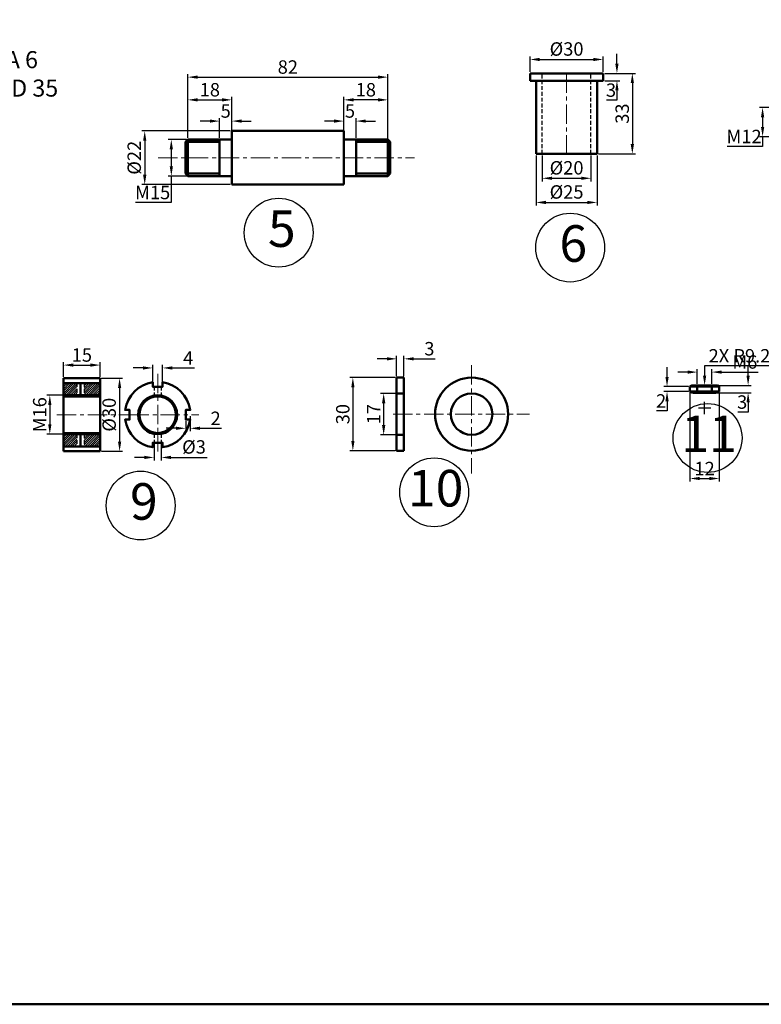
# Model space of a CAD drawing. Units: millimetres. Extents: x -3 to 930, y -425 to 322.
# Tile 2 of 5: x 225 to 529, y -425 to -21. Entities that reach past the tile are written whole.
import ezdxf
from ezdxf import colors
from ezdxf.entities.mleader import LeaderData, LeaderLine
from ezdxf.math import Vec2, Vec3

# ---------------------------------------------------------------- set-up
doc = ezdxf.new("R2010")
doc.units = ezdxf.units.MM
doc.header["$LTSCALE"] = 0.5
doc.linetypes.add('CENTER', pattern=[50.8, 31.75, -6.35, 6.35, -6.35])
doc.linetypes.add('HIDDEN', pattern=[9.525, 6.35, -3.175])
for name, color, linetype, lineweight in [('M-ANNO-SYMB', 3, 'Continuous', 25), ('M-CNTR', 1, 'CENTER', 18), ('M-DIMS', 2, 'Continuous', 25), ('M-HATC', 8, 'Continuous', 18), ('M-HIDN', 4, 'HIDDEN', 25), ('M-OUTL', 7, 'Continuous', 50), ('M-TEXT', 3, 'Continuous', 25)]:
    doc.layers.add(name, color=color, linetype=linetype, lineweight=lineweight)
doc.styles.get("Standard").update_dxf_attribs({"font": 'arial.ttf'})
doc.dimstyles.new('ISO-25', dxfattribs={"dimtxt": 5.5, "dimasz": 4, "dimexe": 1.25, "dimexo": 0.625, "dimtad": 1, "dimtoh": 1, "dimdec": 0, "dimtxsty": 'Standard', "dimcen": 2.5, "dimadec": 0, "dimazin": 0, "dimtfac": 1, "dimtdec": 0, "dimtofl": 0, "dimtmove": 0, "dimatfit": 3, "dimfxl": 1, "dimarcsym": 0})

# ---------------------------------------------------------------- blocks, each defined once
blk = doc.blocks.new('*D49')
at = {"layer": 'Defpoints', "color": 0, "ltscale": 0.5, "transparency": 16777216}
for p in [(311.91, -62.44), (306.91, -69.98), (311.91, -69.98)]:
    blk.add_point(p, dxfattribs=at)
at = {"layer": 'M-DIMS', "color": 0, "lineweight": -2, "ltscale": 0.5, "transparency": 16777216}
for p, q in [((302.91, -62.44), (298.91, -62.44)), ((306.91, -69.36), (306.91, -61.19)), ((311.91, -69.36), (311.91, -61.19)), ((315.91, -62.44), (319.91, -62.44))]:
    blk.add_line(p, q, dxfattribs=at)
at = {"layer": 'M-DIMS', "color": 0, "ltscale": 0.5, "transparency": 16777216}
for points in [[(302.91, -61.77), (302.91, -63.1), (306.91, -62.44)], [(315.91, -61.77), (315.91, -63.1), (311.91, -62.44)]]:
    blk.add_solid(points, dxfattribs=at)
at = {"layer": 'M-DIMS', "color": 0, "ltscale": 0.5, "transparency": 16777216, "insert": (309.41, -59.01), "char_height": 5.5, "attachment_point": 5}
blk.add_mtext('5', dxfattribs=at)
blk = doc.blocks.new('*D50')
at = {"layer": 'Defpoints', "color": 0, "ltscale": 0.5, "transparency": 16777216}
for p in [(311.91, -53.72), (293.91, -69.98), (311.91, -69.98)]:
    blk.add_point(p, dxfattribs=at)
at = {"layer": 'M-DIMS', "color": 0, "lineweight": -2, "ltscale": 0.5, "transparency": 16777216}
for p, q in [((293.91, -69.36), (293.91, -52.47)), ((311.91, -69.36), (311.91, -52.47)), ((297.91, -53.72), (307.91, -53.72))]:
    blk.add_line(p, q, dxfattribs=at)
at = {"layer": 'M-DIMS', "color": 0, "ltscale": 0.5, "transparency": 16777216}
for points in [[(297.91, -53.06), (297.91, -54.39), (293.91, -53.72)], [(307.91, -53.06), (307.91, -54.39), (311.91, -53.72)]]:
    blk.add_solid(points, dxfattribs=at)
at = {"layer": 'M-DIMS', "color": 0, "ltscale": 0.5, "transparency": 16777216, "insert": (302.91, -50.29), "char_height": 5.5, "attachment_point": 5}
blk.add_mtext('18', dxfattribs=at)
blk = doc.blocks.new('*D51')
at = {"layer": 'Defpoints', "color": 0, "ltscale": 0.5, "transparency": 16777216}
for p in [(375.91, -44.4), (293.91, -58.17), (375.91, -70.98)]:
    blk.add_point(p, dxfattribs=at)
at = {"layer": 'M-DIMS', "color": 0, "lineweight": -2, "ltscale": 0.5, "transparency": 16777216}
for p, q in [((293.91, -57.54), (293.91, -43.15)), ((297.91, -44.4), (371.91, -44.4)), ((375.91, -70.36), (375.91, -43.15))]:
    blk.add_line(p, q, dxfattribs=at)
at = {"layer": 'M-DIMS', "color": 0, "ltscale": 0.5, "transparency": 16777216}
for points in [[(297.91, -43.73), (297.91, -45.06), (293.91, -44.4)], [(371.91, -43.73), (371.91, -45.06), (375.91, -44.4)]]:
    blk.add_solid(points, dxfattribs=at)
at = {"layer": 'M-DIMS', "color": 0, "ltscale": 0.5, "transparency": 16777216, "insert": (334.91, -40.96), "char_height": 5.5, "attachment_point": 5}
blk.add_mtext('82', dxfattribs=at)
blk = doc.blocks.new('*D52')
at = {"layer": 'Defpoints', "color": 0, "ltscale": 0.5, "transparency": 16777216}
for p in [(311.91, -66.48), (276.18, -88.48), (311.91, -88.48)]:
    blk.add_point(p, dxfattribs=at)
at = {"layer": 'M-DIMS', "color": 0, "lineweight": -2, "ltscale": 0.5, "transparency": 16777216}
for p, q in [((311.28, -66.48), (274.93, -66.48)), ((276.18, -70.48), (276.18, -84.48)), ((311.28, -88.48), (274.93, -88.48))]:
    blk.add_line(p, q, dxfattribs=at)
at = {"layer": 'M-DIMS', "color": 0, "ltscale": 0.5, "transparency": 16777216}
for points in [[(275.51, -70.48), (276.85, -70.48), (276.18, -66.48)], [(275.51, -84.48), (276.85, -84.48), (276.18, -88.48)]]:
    blk.add_solid(points, dxfattribs=at)
at = {"layer": 'M-DIMS', "color": 0, "ltscale": 0.5, "transparency": 16777216, "insert": (272.59, -77.48), "char_height": 5.5, "attachment_point": 5, "rotation": 90}
blk.add_mtext('%%C22', dxfattribs=at)
blk = doc.blocks.new('*D53')
at = {"layer": 'Defpoints', "color": 0, "ltscale": 0.5, "transparency": 16777216}
for p in [(293.91, -69.98), (287.09, -84.98), (293.91, -84.98)]:
    blk.add_point(p, dxfattribs=at)
at = {"layer": 'M-DIMS', "color": 0, "lineweight": -2, "ltscale": 0.5, "transparency": 16777216}
for p, q in [((293.28, -69.98), (285.84, -69.98)), ((287.09, -73.98), (287.09, -80.98)), ((293.28, -84.98), (285.84, -84.98)), ((287.09, -84.98), (287.09, -95.89)), ((287.09, -95.89), (272.4, -95.89))]:
    blk.add_line(p, q, dxfattribs=at)
at = {"layer": 'M-DIMS', "color": 0, "ltscale": 0.5, "transparency": 16777216}
for points in [[(286.43, -73.98), (287.76, -73.98), (287.09, -69.98)], [(286.43, -80.98), (287.76, -80.98), (287.09, -84.98)]]:
    blk.add_solid(points, dxfattribs=at)
at = {"layer": 'M-DIMS', "color": 0, "ltscale": 0.5, "transparency": 16777216, "insert": (279.43, -92.46), "char_height": 5.5, "width": 8.2937, "attachment_point": 5}
blk.add_mtext('M15', dxfattribs=at)
blk = doc.blocks.new('*D54')
at = {"layer": 'Defpoints', "color": 0, "ltscale": 0.5, "transparency": 16777216}
for p in [(357.91, -62.44), (357.91, -69.98), (362.91, -69.98)]:
    blk.add_point(p, dxfattribs=at)
at = {"layer": 'M-DIMS', "color": 0, "lineweight": -2, "ltscale": 0.5, "transparency": 16777216}
for p, q in [((353.91, -62.44), (349.91, -62.44)), ((357.91, -69.36), (357.91, -61.19)), ((362.91, -69.36), (362.91, -61.19)), ((366.91, -62.44), (370.91, -62.44))]:
    blk.add_line(p, q, dxfattribs=at)
at = {"layer": 'M-DIMS', "color": 0, "ltscale": 0.5, "transparency": 16777216}
for points in [[(353.91, -61.77), (353.91, -63.1), (357.91, -62.44)], [(366.91, -61.77), (366.91, -63.1), (362.91, -62.44)]]:
    blk.add_solid(points, dxfattribs=at)
at = {"layer": 'M-DIMS', "color": 0, "ltscale": 0.5, "transparency": 16777216, "insert": (360.41, -59.01), "char_height": 5.5, "attachment_point": 5}
blk.add_mtext('5', dxfattribs=at)
blk = doc.blocks.new('*D55')
at = {"layer": 'Defpoints', "color": 0, "ltscale": 0.5, "transparency": 16777216}
for p in [(357.91, -53.72), (357.91, -69.98), (375.91, -69.98)]:
    blk.add_point(p, dxfattribs=at)
at = {"layer": 'M-DIMS', "color": 0, "lineweight": -2, "ltscale": 0.5, "transparency": 16777216}
for p, q in [((357.91, -69.36), (357.91, -52.47)), ((375.91, -69.36), (375.91, -52.47)), ((371.91, -53.72), (361.91, -53.72))]:
    blk.add_line(p, q, dxfattribs=at)
at = {"layer": 'M-DIMS', "color": 0, "ltscale": 0.5, "transparency": 16777216}
for points in [[(361.91, -53.06), (361.91, -54.39), (357.91, -53.72)], [(371.91, -53.06), (371.91, -54.39), (375.91, -53.72)]]:
    blk.add_solid(points, dxfattribs=at)
at = {"layer": 'M-DIMS', "color": 0, "ltscale": 0.5, "transparency": 16777216, "insert": (366.91, -50.29), "char_height": 5.5, "attachment_point": 5}
blk.add_mtext('18', dxfattribs=at)
blk = doc.blocks.new('*D56')
at = {"layer": 'Defpoints', "color": 0, "ltscale": 0.5, "transparency": 16777216}
for p in [(464.29, -42.87), (464.29, -45.87), (469.95, -45.87)]:
    blk.add_point(p, dxfattribs=at)
at = {"layer": 'M-DIMS', "color": 0, "lineweight": -2, "ltscale": 0.5, "transparency": 16777216}
for p, q in [((469.95, -38.87), (469.95, -34.87)), ((464.92, -42.87), (471.2, -42.87)), ((464.92, -45.87), (471.2, -45.87)), ((469.95, -49.87), (469.95, -53.87)), ((469.95, -53.87), (465.72, -53.87))]:
    blk.add_line(p, q, dxfattribs=at)
at = {"layer": 'M-DIMS', "color": 0, "ltscale": 0.5, "transparency": 16777216}
for points in [[(469.28, -38.87), (470.62, -38.87), (469.95, -42.87)], [(469.28, -49.87), (470.62, -49.87), (469.95, -45.87)]]:
    blk.add_solid(points, dxfattribs=at)
at = {"layer": 'M-DIMS', "color": 0, "ltscale": 0.5, "transparency": 16777216, "insert": (467.52, -50.43), "char_height": 5.5, "attachment_point": 5}
blk.add_mtext('3', dxfattribs=at)
blk = doc.blocks.new('*D57')
at = {"layer": 'Defpoints', "color": 0, "ltscale": 0.5, "transparency": 16777216}
for p in [(464.29, -42.87), (461.79, -75.87), (476.27, -75.87)]:
    blk.add_point(p, dxfattribs=at)
at = {"layer": 'M-DIMS', "color": 0, "lineweight": -2, "ltscale": 0.5, "transparency": 16777216}
for p, q in [((464.92, -42.87), (477.52, -42.87)), ((476.27, -46.87), (476.27, -71.87)), ((462.42, -75.87), (477.52, -75.87))]:
    blk.add_line(p, q, dxfattribs=at)
at = {"layer": 'M-DIMS', "color": 0, "ltscale": 0.5, "transparency": 16777216}
for points in [[(475.6, -46.87), (476.94, -46.87), (476.27, -42.87)], [(475.6, -71.87), (476.94, -71.87), (476.27, -75.87)]]:
    blk.add_solid(points, dxfattribs=at)
at = {"layer": 'M-DIMS', "color": 0, "ltscale": 0.5, "transparency": 16777216, "insert": (472.83, -59.37), "char_height": 5.5, "attachment_point": 5, "rotation": 90}
blk.add_mtext('33', dxfattribs=at)
blk = doc.blocks.new('*D58')
at = {"layer": 'Defpoints', "color": 0, "ltscale": 0.5, "transparency": 16777216}
for p in [(439.29, -75.87), (459.29, -75.87), (459.29, -85.91)]:
    blk.add_point(p, dxfattribs=at)
at = {"layer": 'M-DIMS', "color": 0, "lineweight": -2, "ltscale": 0.5, "transparency": 16777216}
for p, q in [((439.29, -76.49), (439.29, -87.16)), ((459.29, -76.49), (459.29, -87.16)), ((443.29, -85.91), (455.29, -85.91))]:
    blk.add_line(p, q, dxfattribs=at)
at = {"layer": 'M-DIMS', "color": 0, "ltscale": 0.5, "transparency": 16777216}
for points in [[(443.29, -85.24), (443.29, -86.57), (439.29, -85.91)], [(455.29, -85.24), (455.29, -86.57), (459.29, -85.91)]]:
    blk.add_solid(points, dxfattribs=at)
at = {"layer": 'M-DIMS', "color": 0, "ltscale": 0.5, "transparency": 16777216, "insert": (449.29, -82.32), "char_height": 5.5, "attachment_point": 5}
blk.add_mtext('%%C20', dxfattribs=at)
blk = doc.blocks.new('*D59')
at = {"layer": 'Defpoints', "color": 0, "ltscale": 0.5, "transparency": 16777216}
for p in [(436.79, -75.87), (461.79, -75.87), (461.79, -95.82)]:
    blk.add_point(p, dxfattribs=at)
at = {"layer": 'M-DIMS', "color": 0, "lineweight": -2, "ltscale": 0.5, "transparency": 16777216}
for p, q in [((436.79, -76.49), (436.79, -97.07)), ((461.79, -76.49), (461.79, -97.07)), ((440.79, -95.82), (457.79, -95.82))]:
    blk.add_line(p, q, dxfattribs=at)
at = {"layer": 'M-DIMS', "color": 0, "ltscale": 0.5, "transparency": 16777216}
for points in [[(440.79, -95.15), (440.79, -96.49), (436.79, -95.82)], [(457.79, -95.15), (457.79, -96.49), (461.79, -95.82)]]:
    blk.add_solid(points, dxfattribs=at)
at = {"layer": 'M-DIMS', "color": 0, "ltscale": 0.5, "transparency": 16777216, "insert": (449.29, -92.23), "char_height": 5.5, "attachment_point": 5}
blk.add_mtext('%%C25', dxfattribs=at)
blk = doc.blocks.new('*D60')
at = {"layer": 'Defpoints', "color": 0, "ltscale": 0.5, "transparency": 16777216}
for p in [(464.29, -37.15), (434.29, -42.87), (464.29, -42.87)]:
    blk.add_point(p, dxfattribs=at)
at = {"layer": 'M-DIMS', "color": 0, "lineweight": -2, "ltscale": 0.5, "transparency": 16777216}
for p, q in [((434.29, -42.24), (434.29, -35.9)), ((464.29, -42.24), (464.29, -35.9)), ((438.29, -37.15), (460.29, -37.15))]:
    blk.add_line(p, q, dxfattribs=at)
at = {"layer": 'M-DIMS', "color": 0, "ltscale": 0.5, "transparency": 16777216}
for points in [[(438.29, -36.48), (438.29, -37.82), (434.29, -37.15)], [(460.29, -36.48), (460.29, -37.82), (464.29, -37.15)]]:
    blk.add_solid(points, dxfattribs=at)
at = {"layer": 'M-DIMS', "color": 0, "ltscale": 0.5, "transparency": 16777216, "insert": (449.29, -33.56), "char_height": 5.5, "attachment_point": 5}
blk.add_mtext('%%C30', dxfattribs=at)
blk = doc.blocks.new('*D66')
at = {"layer": 'Defpoints', "color": 0, "ltscale": 0.5, "transparency": 16777216}
for p in [(257.89, -167.94), (257.89, -197.94), (265.87, -197.94)]:
    blk.add_point(p, dxfattribs=at)
at = {"layer": 'M-DIMS', "color": 0, "lineweight": -2, "ltscale": 0.5, "transparency": 16777216}
for p, q in [((258.51, -167.94), (267.12, -167.94)), ((265.87, -171.94), (265.87, -193.94)), ((258.51, -197.94), (267.12, -197.94))]:
    blk.add_line(p, q, dxfattribs=at)
at = {"layer": 'M-DIMS', "color": 0, "ltscale": 0.5, "transparency": 16777216}
for points in [[(265.21, -171.94), (266.54, -171.94), (265.87, -167.94)], [(265.21, -193.94), (266.54, -193.94), (265.87, -197.94)]]:
    blk.add_solid(points, dxfattribs=at)
at = {"layer": 'M-DIMS', "color": 0, "ltscale": 0.5, "transparency": 16777216, "insert": (262.29, -182.94), "char_height": 5.5, "attachment_point": 5, "rotation": 90}
blk.add_mtext('%%C30', dxfattribs=at)
blk = doc.blocks.new('*D67')
at = {"layer": 'Defpoints', "color": 0, "ltscale": 0.5, "transparency": 16777216}
for p in [(257.89, -162.57), (242.89, -167.94), (257.89, -167.94)]:
    blk.add_point(p, dxfattribs=at)
at = {"layer": 'M-DIMS', "color": 0, "lineweight": -2, "ltscale": 0.5, "transparency": 16777216}
for p, q in [((242.89, -167.32), (242.89, -161.32)), ((257.89, -167.32), (257.89, -161.32)), ((246.89, -162.57), (253.89, -162.57))]:
    blk.add_line(p, q, dxfattribs=at)
at = {"layer": 'M-DIMS', "color": 0, "ltscale": 0.5, "transparency": 16777216}
for points in [[(246.89, -161.9), (246.89, -163.24), (242.89, -162.57)], [(253.89, -161.9), (253.89, -163.24), (257.89, -162.57)]]:
    blk.add_solid(points, dxfattribs=at)
at = {"layer": 'M-DIMS', "color": 0, "ltscale": 0.5, "transparency": 16777216, "insert": (250.39, -159.14), "char_height": 5.5, "attachment_point": 5}
blk.add_mtext('15', dxfattribs=at)
blk = doc.blocks.new('*D68')
at = {"layer": 'Defpoints', "color": 0, "ltscale": 0.5, "transparency": 16777216}
for p in [(242.89, -174.94), (237.24, -190.94), (242.89, -190.94)]:
    blk.add_point(p, dxfattribs=at)
at = {"layer": 'M-DIMS', "color": 0, "lineweight": -2, "ltscale": 0.5, "transparency": 16777216}
for p, q in [((242.26, -174.94), (235.99, -174.94)), ((237.24, -178.94), (237.24, -186.94)), ((242.26, -190.94), (235.99, -190.94))]:
    blk.add_line(p, q, dxfattribs=at)
at = {"layer": 'M-DIMS', "color": 0, "ltscale": 0.5, "transparency": 16777216}
for points in [[(236.57, -178.94), (237.9, -178.94), (237.24, -174.94)], [(236.57, -186.94), (237.9, -186.94), (237.24, -190.94)]]:
    blk.add_solid(points, dxfattribs=at)
at = {"layer": 'M-DIMS', "color": 0, "ltscale": 0.5, "transparency": 16777216, "insert": (233.8, -182.94), "char_height": 5.5, "attachment_point": 5, "rotation": 90}
blk.add_mtext('M16', dxfattribs=at)
blk = doc.blocks.new('*D69')
at = {"layer": 'Defpoints', "color": 0, "ltscale": 0.5, "transparency": 16777216}
for p in [(283.49, -163.74), (279.49, -171.44), (283.49, -171.44)]:
    blk.add_point(p, dxfattribs=at)
at = {"layer": 'M-DIMS', "color": 0, "lineweight": -2, "ltscale": 0.5, "transparency": 16777216}
for p, q in [((275.49, -163.74), (271.49, -163.74)), ((279.49, -170.82), (279.49, -162.49)), ((283.49, -170.82), (283.49, -162.49)), ((287.49, -163.74), (296.55, -163.74))]:
    blk.add_line(p, q, dxfattribs=at)
at = {"layer": 'M-DIMS', "color": 0, "ltscale": 0.5, "transparency": 16777216}
for points in [[(275.49, -163.08), (275.49, -164.41), (279.49, -163.74)], [(287.49, -163.08), (287.49, -164.41), (283.49, -163.74)]]:
    blk.add_solid(points, dxfattribs=at)
at = {"layer": 'M-DIMS', "color": 0, "ltscale": 0.5, "transparency": 16777216, "insert": (294.02, -160.37), "char_height": 5.5, "attachment_point": 5}
blk.add_mtext('4', dxfattribs=at)
blk = doc.blocks.new('*D70')
at = {"layer": 'Defpoints', "color": 0, "ltscale": 0.5, "transparency": 16777216}
for p in [(279.99, -194.44), (282.99, -194.44), (282.99, -200.46)]:
    blk.add_point(p, dxfattribs=at)
at = {"layer": 'M-DIMS', "color": 0, "lineweight": -2, "ltscale": 0.5, "transparency": 16777216}
for p, q in [((279.99, -195.07), (279.99, -201.71)), ((282.99, -195.07), (282.99, -201.71)), ((275.99, -200.46), (271.99, -200.46)), ((286.99, -200.46), (301.83, -200.46))]:
    blk.add_line(p, q, dxfattribs=at)
at = {"layer": 'M-DIMS', "color": 0, "ltscale": 0.5, "transparency": 16777216}
for points in [[(275.99, -199.79), (275.99, -201.13), (279.99, -200.46)], [(286.99, -199.79), (286.99, -201.13), (282.99, -200.46)]]:
    blk.add_solid(points, dxfattribs=at)
at = {"layer": 'M-DIMS', "color": 0, "ltscale": 0.5, "transparency": 16777216, "insert": (296.41, -196.87), "char_height": 5.5, "attachment_point": 5}
blk.add_mtext('%%C3', dxfattribs=at)
blk = doc.blocks.new('*D71')
at = {"layer": 'Defpoints', "color": 0, "ltscale": 0.5, "transparency": 16777216}
for p in [(292.99, -184.94), (294.84, -182.94), (294.84, -188.5)]:
    blk.add_point(p, dxfattribs=at)
at = {"layer": 'M-DIMS', "color": 0, "lineweight": -2, "ltscale": 0.5, "transparency": 16777216}
for p, q in [((292.99, -185.57), (292.99, -189.75)), ((294.84, -183.57), (294.84, -189.75)), ((288.99, -188.5), (284.99, -188.5)), ((298.84, -188.5), (307.74, -188.5))]:
    blk.add_line(p, q, dxfattribs=at)
at = {"layer": 'M-DIMS', "color": 0, "ltscale": 0.5, "transparency": 16777216}
for points in [[(288.99, -187.83), (288.99, -189.17), (292.99, -188.5)], [(298.84, -187.83), (298.84, -189.17), (294.84, -188.5)]]:
    blk.add_solid(points, dxfattribs=at)
at = {"layer": 'M-DIMS', "color": 0, "ltscale": 0.5, "transparency": 16777216, "insert": (305.29, -185.12), "char_height": 5.5, "attachment_point": 5}
blk.add_mtext('2', dxfattribs=at)
blk = doc.blocks.new('*D75')
at = {"layer": 'Defpoints', "color": 0, "ltscale": 0.5, "transparency": 16777216}
for p in [(539.21, -56.85), (529.72, -68.85), (539.21, -68.85)]:
    blk.add_point(p, dxfattribs=at)
at = {"layer": 'M-DIMS', "color": 0, "lineweight": -2, "ltscale": 0.5, "transparency": 16777216}
for p, q in [((538.59, -56.85), (528.47, -56.85)), ((529.72, -60.85), (529.72, -64.85)), ((538.59, -68.85), (528.47, -68.85)), ((529.72, -68.85), (529.72, -72.85)), ((529.72, -72.85), (515.13, -72.85))]:
    blk.add_line(p, q, dxfattribs=at)
at = {"layer": 'M-DIMS', "color": 0, "ltscale": 0.5, "transparency": 16777216}
for points in [[(529.06, -60.85), (530.39, -60.85), (529.72, -56.85)], [(529.06, -64.85), (530.39, -64.85), (529.72, -68.85)]]:
    blk.add_solid(points, dxfattribs=at)
at = {"layer": 'M-DIMS', "color": 0, "ltscale": 0.5, "transparency": 16777216, "insert": (522.11, -69.46), "char_height": 5.5, "attachment_point": 5}
blk.add_mtext('M12', dxfattribs=at)
blk = doc.blocks.new('*D77')
at = {"layer": 'Defpoints', "color": 0, "ltscale": 0.5, "transparency": 16777216}
for p in [(379.55, -167.7), (361.59, -197.7), (379.55, -197.7)]:
    blk.add_point(p, dxfattribs=at)
at = {"layer": 'M-DIMS', "color": 0, "lineweight": -2, "ltscale": 0.5, "transparency": 16777216}
for p, q in [((378.93, -167.7), (360.34, -167.7)), ((361.59, -171.7), (361.59, -193.7)), ((378.93, -197.7), (360.34, -197.7))]:
    blk.add_line(p, q, dxfattribs=at)
at = {"layer": 'M-DIMS', "color": 0, "ltscale": 0.5, "transparency": 16777216}
for points in [[(360.93, -171.7), (362.26, -171.7), (361.59, -167.7)], [(360.93, -193.7), (362.26, -193.7), (361.59, -197.7)]]:
    blk.add_solid(points, dxfattribs=at)
at = {"layer": 'M-DIMS', "color": 0, "ltscale": 0.5, "transparency": 16777216, "insert": (358.16, -182.7), "char_height": 5.5, "attachment_point": 5, "rotation": 90}
blk.add_mtext('30', dxfattribs=at)
blk = doc.blocks.new('*D78')
at = {"layer": 'Defpoints', "color": 0, "ltscale": 0.5, "transparency": 16777216}
for p in [(379.55, -174.2), (374.23, -191.2), (379.55, -191.2)]:
    blk.add_point(p, dxfattribs=at)
at = {"layer": 'M-DIMS', "color": 0, "lineweight": -2, "ltscale": 0.5, "transparency": 16777216}
for p, q in [((378.93, -174.2), (372.98, -174.2)), ((374.23, -178.2), (374.23, -187.2)), ((378.93, -191.2), (372.98, -191.2))]:
    blk.add_line(p, q, dxfattribs=at)
at = {"layer": 'M-DIMS', "color": 0, "ltscale": 0.5, "transparency": 16777216}
for points in [[(373.56, -178.2), (374.9, -178.2), (374.23, -174.2)], [(373.56, -187.2), (374.9, -187.2), (374.23, -191.2)]]:
    blk.add_solid(points, dxfattribs=at)
at = {"layer": 'M-DIMS', "color": 0, "ltscale": 0.5, "transparency": 16777216, "insert": (370.84, -182.7), "char_height": 5.5, "attachment_point": 5, "rotation": 90}
blk.add_mtext('17', dxfattribs=at)
blk = doc.blocks.new('*D79')
at = {"layer": 'Defpoints', "color": 0, "ltscale": 0.5, "transparency": 16777216}
for p in [(382.55, -160), (379.55, -167.7), (382.55, -167.7)]:
    blk.add_point(p, dxfattribs=at)
at = {"layer": 'M-DIMS', "color": 0, "lineweight": -2, "ltscale": 0.5, "transparency": 16777216}
for p, q in [((375.55, -160), (371.55, -160)), ((379.55, -167.08), (379.55, -158.75)), ((382.55, -167.08), (382.55, -158.75)), ((386.55, -160), (395.4, -160))]:
    blk.add_line(p, q, dxfattribs=at)
at = {"layer": 'M-DIMS', "color": 0, "ltscale": 0.5, "transparency": 16777216}
for points in [[(375.55, -159.33), (375.55, -160.67), (379.55, -160)], [(386.55, -159.33), (386.55, -160.67), (382.55, -160)]]:
    blk.add_solid(points, dxfattribs=at)
at = {"layer": 'M-DIMS', "color": 0, "ltscale": 0.5, "transparency": 16777216, "insert": (392.98, -156.56), "char_height": 5.5, "attachment_point": 5}
blk.add_mtext('3', dxfattribs=at)
blk = doc.blocks.new('*D80')
at = {"layer": 'Defpoints', "color": 0, "ltscale": 0.5, "transparency": 16777216}
for p in [(508.93, -165.44), (502.93, -170.89), (508.93, -170.89)]:
    blk.add_point(p, dxfattribs=at)
at = {"layer": 'M-DIMS', "color": 0, "lineweight": -2, "ltscale": 0.5, "transparency": 16777216}
for p, q in [((498.93, -165.44), (494.93, -165.44)), ((502.93, -170.26), (502.93, -164.19)), ((508.93, -170.26), (508.93, -164.19)), ((512.93, -165.44), (527.93, -165.44))]:
    blk.add_line(p, q, dxfattribs=at)
at = {"layer": 'M-DIMS', "color": 0, "ltscale": 0.5, "transparency": 16777216}
for points in [[(498.93, -164.78), (498.93, -166.11), (502.93, -165.44)], [(512.93, -164.78), (512.93, -166.11), (508.93, -165.44)]]:
    blk.add_solid(points, dxfattribs=at)
at = {"layer": 'M-DIMS', "color": 0, "ltscale": 0.5, "transparency": 16777216, "insert": (522.43, -162.01), "char_height": 5.5, "attachment_point": 5}
blk.add_mtext('M6', dxfattribs=at)
blk = doc.blocks.new('BALLOON')
at = {"ltscale": 0.5}
blk.add_circle((198.15, 8.03), 14.13, dxfattribs=at)
blk = doc.blocks.new('*D86')
at = {"layer": 'Defpoints', "color": 0, "ltscale": 0.5, "transparency": 16777216}
for p in [(499.93, -173.39), (511.93, -173.39), (511.93, -209.11)]:
    blk.add_point(p, dxfattribs=at)
at = {"layer": 'M-DIMS', "color": 0, "lineweight": -2, "ltscale": 0.5, "transparency": 16777216}
for p, q in [((499.93, -174.01), (499.93, -210.36)), ((511.93, -174.01), (511.93, -210.36)), ((503.93, -209.11), (507.93, -209.11))]:
    blk.add_line(p, q, dxfattribs=at)
at = {"layer": 'M-DIMS', "color": 0, "ltscale": 0.5, "transparency": 16777216}
for points in [[(503.93, -208.45), (503.93, -209.78), (499.93, -209.11)], [(507.93, -208.45), (507.93, -209.78), (511.93, -209.11)]]:
    blk.add_solid(points, dxfattribs=at)
at = {"layer": 'M-DIMS', "color": 0, "ltscale": 0.5, "transparency": 16777216, "insert": (505.93, -205.73), "char_height": 5.5, "attachment_point": 5}
blk.add_mtext('12', dxfattribs=at)
blk = doc.blocks.new('*D87')
at = {"layer": 'Defpoints', "color": 0, "ltscale": 0.5, "transparency": 16777216}
for p in [(508.93, -170.89), (508.93, -173.89), (523.78, -173.89)]:
    blk.add_point(p, dxfattribs=at)
at = {"layer": 'M-DIMS', "color": 0, "lineweight": -2, "ltscale": 0.5, "transparency": 16777216}
for p, q in [((523.78, -166.89), (523.78, -162.89)), ((509.55, -170.89), (525.03, -170.89)), ((509.55, -173.89), (525.03, -173.89)), ((523.78, -177.89), (523.78, -181.89)), ((523.78, -181.89), (519.55, -181.89))]:
    blk.add_line(p, q, dxfattribs=at)
at = {"layer": 'M-DIMS', "color": 0, "ltscale": 0.5, "transparency": 16777216}
for points in [[(523.11, -166.89), (524.45, -166.89), (523.78, -170.89)], [(523.11, -177.89), (524.45, -177.89), (523.78, -173.89)]]:
    blk.add_solid(points, dxfattribs=at)
at = {"layer": 'M-DIMS', "color": 0, "ltscale": 0.5, "transparency": 16777216, "insert": (521.35, -178.45), "char_height": 5.5, "attachment_point": 5}
blk.add_mtext('3', dxfattribs=at)
blk = doc.blocks.new('*D88')
at = {"layer": 'Defpoints', "color": 0, "ltscale": 0.5, "transparency": 16777216}
for p in [(490.51, -173.39), (499.93, -171.39), (499.93, -173.39)]:
    blk.add_point(p, dxfattribs=at)
at = {"layer": 'M-DIMS', "color": 0, "lineweight": -2, "ltscale": 0.5, "transparency": 16777216}
for p, q in [((490.51, -167.39), (490.51, -163.39)), ((499.3, -171.39), (489.26, -171.39)), ((499.3, -173.39), (489.26, -173.39)), ((490.51, -177.39), (490.51, -181.39)), ((490.51, -181.39), (486.25, -181.39))]:
    blk.add_line(p, q, dxfattribs=at)
at = {"layer": 'M-DIMS', "color": 0, "ltscale": 0.5, "transparency": 16777216}
for points in [[(489.85, -167.39), (491.18, -167.39), (490.51, -171.39)], [(489.85, -177.39), (491.18, -177.39), (490.51, -173.39)]]:
    blk.add_solid(points, dxfattribs=at)
at = {"layer": 'M-DIMS', "color": 0, "ltscale": 0.5, "transparency": 16777216, "insert": (488.07, -178), "char_height": 5.5, "attachment_point": 5}
blk.add_mtext('2', dxfattribs=at)
blk = doc.blocks.new('*D95')
at = {"layer": 'Defpoints', "color": 0, "ltscale": 0.5, "transparency": 16777216}
for p in [(505.93, -170.89), (505.93, -180.14)]:
    blk.add_point(p, dxfattribs=at)
at = {"layer": 'M-DIMS', "color": 0, "lineweight": -2, "ltscale": 0.5, "transparency": 16777216}
for p, q in [((538.06, -162.89), (505.93, -162.89)), ((505.93, -162.89), (505.93, -166.89)), ((505.93, -182.64), (505.93, -177.64)), ((503.43, -180.14), (508.43, -180.14))]:
    blk.add_line(p, q, dxfattribs=at)
at = {"layer": 'M-DIMS', "color": 0, "ltscale": 0.5, "transparency": 16777216}
blk.add_solid([(505.26, -166.89), (506.6, -166.89), (505.93, -170.89)], dxfattribs=at)
at = {"layer": 'M-DIMS', "color": 0, "ltscale": 0.5, "transparency": 16777216, "insert": (522.31, -159.46), "char_height": 5.5, "attachment_point": 5}
blk.add_mtext('2X R9.25', dxfattribs=at)

msp = doc.modelspace()

# ---------------------------------------------------------------- hatches: boundary and pattern name
at = {"layer": 'M-HATC', "ltscale": 0.5}
h = msp.add_hatch(dxfattribs=at)
h.set_pattern_fill('ANSI31', color=256, scale=0.2)
h.set_pattern_definition([(45, (-144.14956, -22.4151), (-0.4490128, 0.4490128), [])])
h.paths.add_polyline_path([(248.3864, -195.9445), (248.3864, -190.9445), (242.8864, -190.9445), (242.8864, -195.9445)])
h.paths.add_polyline_path([(251.3864, -195.9445), (257.8864, -195.9445), (257.8864, -190.9445), (251.3864, -190.9445)])
h.paths.add_polyline_path([(248.3864, -169.9445), (242.8864, -169.9445), (242.8864, -174.9445), (248.3864, -174.9445)])
h.paths.add_polyline_path([(251.3864, -174.9445), (257.8864, -174.9445), (257.8864, -169.9445), (251.3864, -169.9445)])

# ---------------------------------------------------------------- linework, layer by layer
at = {"layer": 'M-CNTR', "ltscale": 0.5}
for p, q in [((449.2936, -42.8663), (449.2936, -75.8663)), ((281.632, -77.4806), (386.9294, -77.4806)), ((410.3237, -162.602), (410.3237, -207.1161)), ((281.4926, -166.1236), (281.4926, -198.063)), ((378.1018, -182.7009), (434.1032, -182.7009))]:
    msp.add_line(p, q, dxfattribs=at)
msp.add_lwpolyline([(240.101, -182.9445), (269.9926, -182.9445), (298.4404, -182.9445)], dxfattribs=at)
at = {"layer": 'M-HIDN', "ltscale": 0.5}
for p, q in [((439.2936, -75.8663), (439.2936, -42.8663)), ((459.2936, -75.8663), (459.2936, -42.8663)), ((248.3864, -169.9445), (248.3864, -174.9445)), ((251.3864, -169.9445), (251.3864, -174.9445)), ((279.9926, -171.4445), (279.9926, -175.0863)), ((282.9926, -171.4445), (282.9926, -175.0863)), ((248.3864, -190.9445), (248.3864, -195.9445)), ((251.3864, -190.9445), (251.3864, -195.9445)), ((279.9926, -190.8026), (279.9926, -194.4445)), ((282.9926, -190.8026), (282.9926, -194.4445))]:
    msp.add_line(p, q, dxfattribs=at)
at = {"layer": 'M-OUTL', "ltscale": 0.5}
for p, q in [((434.2936, -42.8663), (464.2936, -42.8663)), ((434.2936, -45.8663), (434.2936, -42.8663)), ((464.2936, -42.8663), (464.2936, -45.8663)), ((461.7936, -45.8663), (434.2936, -45.8663)), ((436.7936, -75.8663), (436.7936, -45.8663)), ((464.2936, -45.8663), (461.7936, -45.8663)), ((461.7936, -45.8663), (461.7936, -75.8663)), ((311.9051, -66.4806), (357.9051, -66.4806)), ((311.9051, -88.4806), (311.9051, -66.4806)), ((357.9051, -66.4806), (357.9051, -88.4806)), ((293.9051, -69.9806), (292.9051, -70.9806)), ((306.9051, -70.9806), (292.9051, -70.9806)), ((292.9051, -70.9806), (292.9051, -83.9806)), ((311.9051, -69.9806), (293.9051, -69.9806)), ((293.9051, -69.9806), (293.9051, -84.9806)), ((306.9051, -69.9806), (306.9051, -84.9806)), ((357.9051, -69.9806), (375.9051, -69.9806)), ((357.9051, -69.9806), (357.9051, -84.9806)), ((362.9051, -69.9806), (362.9051, -84.9806)), ((362.9051, -70.9806), (376.9051, -70.9806)), ((375.9051, -69.9806), (375.9051, -84.9806)), ((375.9051, -69.9806), (376.9051, -70.9806)), ((376.9051, -70.9806), (376.9051, -83.9806)), ((461.7936, -75.8663), (436.7936, -75.8663)), ((292.9051, -83.9806), (306.9051, -83.9806)), ((293.9051, -84.9806), (292.9051, -83.9806)), ((376.9051, -83.9806), (362.9051, -83.9806)), ((375.9051, -84.9806), (376.9051, -83.9806)), ((293.9051, -84.9806), (311.9051, -84.9806)), ((357.9051, -88.4806), (311.9051, -88.4806)), ((375.9051, -84.9806), (357.9051, -84.9806)), ((257.8864, -167.9445), (242.8864, -167.9445)), ((242.8864, -167.9445), (242.8864, -197.9445)), ((257.8864, -182.9445), (257.8864, -167.9445)), ((379.553, -197.7009), (379.553, -167.7009)), ((379.553, -167.7009), (382.553, -167.7009)), ((382.553, -167.7009), (382.553, -197.7009)), ((257.8864, -169.9445), (242.8864, -169.9445)), ((249.8864, -169.9445), (249.8864, -174.9445)), ((499.9288, -173.3883), (499.9288, -171.3883)), ((499.9288, -171.3883), (511.9288, -171.3883)), ((499.9288, -173.3883), (511.9288, -173.3883)), ((501.2381, -170.8883), (510.5264, -170.8883)), ((502.9288, -173.8883), (502.9288, -170.8883)), ((508.9288, -170.8883), (508.9288, -173.8883)), ((511.9288, -171.3883), (511.9288, -173.3883)), ((242.8864, -174.9445), (257.8864, -174.9445)), ((242.8864, -175.4445), (257.8864, -175.4445)), ((382.553, -174.2009), (379.553, -174.2009)), ((510.5264, -173.8883), (501.2381, -173.8883)), ((257.8864, -197.9445), (257.8864, -182.9445)), ((242.8864, -190.4445), (257.8864, -190.4445)), ((242.8864, -190.9445), (257.8864, -190.9445)), ((249.8864, -190.9445), (249.8864, -195.9445)), ((382.553, -191.2009), (379.553, -191.2009)), ((242.8864, -195.9445), (257.8864, -195.9445)), ((242.8864, -197.9445), (257.8864, -197.9445)), ((382.553, -197.7009), (379.553, -197.7009))]:
    msp.add_line(p, q, dxfattribs=at)
msp.add_lwpolyline([(-2.6134, 321.6785), (929.6113, 321.6785), (929.6113, -424.8872), (-2.6134, -424.8872)], close=True, dxfattribs=at)
msp.add_lwpolyline([(279.4926, -169.5934, 0.32956068), (268.1416, -180.9445), (269.9926, -180.9445), (269.9926, -184.9445), (268.1416, -184.9445, 0.32956068), (279.4926, -196.2955), (279.4926, -194.4445), (283.4926, -194.4445), (283.4926, -196.2955, 0.32956068), (294.8437, -184.9445), (292.9926, -184.9445), (292.9926, -180.9445), (294.8437, -180.9445, 0.32956068), (283.4926, -169.5934), (283.4926, -171.4445), (279.4926, -171.4445)], format="xyb", close=True, dxfattribs=at)
for centre, radius in [((410.3237, -182.7009), 15), ((281.4926, -182.9445), 8), ((281.4926, -182.9445), 7.5), ((410.3237, -182.7009), 8.5)]:
    msp.add_circle(centre, radius, dxfattribs=at)
for centre, radius, start, end in [((501.4288, -173.3519), 2.471, 52.624027, 127.375973), ((501.4288, -171.4246), 2.471, 232.624027, 307.375973), ((505.9288, -180.1383), 9.25, 71.075356, 108.924644), ((505.9288, -164.6383), 9.25, 251.075356, 288.924644), ((510.4288, -173.3787), 2.4924, 52.998632, 127.001368), ((510.4288, -171.3978), 2.4924, 232.998632, 307.001368)]:
    msp.add_arc(centre, radius, start, end, dxfattribs=at)

# ---------------------------------------------------------------- block references
at = {"layer": 'M-ANNO-SYMB'}
for p in [(133.0023, -116.2674), (252.6087, -122.3807), (309.0006, -200.5152), (196.8154, -222.8202), (76.3879, -228.2417)]:
    msp.add_blockref('BALLOON', p, dxfattribs=at)

# ---------------------------------------------------------------- texts
at = {"layer": 'M-TEXT', "ltscale": 0.5, "char_height": 15, "attachment_point": 1}
for s, insert in [('5', (326.7541, -99.059)), ('6', (446.3605, -105.1723)), ('11', (496.416, -183.2844)), ('10', (384.2308, -205.5894)), ('9', (270.1397, -211.0333))]:
    msp.add_mtext_dynamic_manual_height_columns(s, width=15, gutter_width=12.5, heights=[0], dxfattribs=dict(at, insert=insert))

# ---------------------------------------------------------------- dimensions: what is measured, and where the dimension line sits
at = {"layer": 'M-DIMS', "ltscale": 0.5}
for base, p1, p2, text, picture, middle in [((464.2936, -37.1509), (434.2936, -42.8663), (464.2936, -42.8663), '%%C<>', '*D60', (449.2936, -33.564)), ((461.7936, -95.8206), (436.7936, -75.8663), (461.7936, -75.8663), '%%C<>', '*D59', (449.2936, -92.2337)), ((459.2936, -85.9062), (439.2936, -75.8663), (459.2936, -75.8663), '%%C<>', '*D58', (449.2936, -82.3192)), ((508.9288, -165.443), (502.9288, -170.8883), (508.9288, -170.8883), 'M<>', '*D80', (522.4292, -162.0099)), ((282.9926, -200.4587), (279.9926, -194.4445), (282.9926, -194.4445), '%%C<>', '*D70', (296.4123, -196.8717))]:
    dim = msp.add_linear_dim(base=base, p1=p1, p2=p2, text=text, dimstyle='ISO-25', override={"dimclrd": 0, "dimclre": 0, "dimclrt": 0}, dxfattribs=at)
    dim.commit()
    dim.dimension.update_dxf_attribs({"geometry": picture, "text_midpoint": middle})
for base, p1, p2, angle, override, picture, middle in [((469.9498, -45.8663), (464.2936, -42.8663), (464.2936, -45.8663), 90, {"dimclrd": 0, "dimclre": 0, "dimclrt": 0}, '*D56', (467.524, -50.4313)), ((476.2695, -75.8663), (464.2936, -42.8663), (461.7936, -75.8663), 90, {"dimclrd": 0, "dimclre": 0, "dimclrt": 0}, '*D57', (472.8345, -59.3663)), ((357.9051, -53.7239), (375.9051, -69.9806), (357.9051, -69.9806), 180, {"dimclrd": 0, "dimclre": 0, "dimclrt": 0}, '*D55', (366.9051, -50.2907)), ((357.9051, -62.4362), (362.9051, -69.9806), (357.9051, -69.9806), 180, {"dimclrd": 0, "dimclre": 0, "dimclrt": 0}, '*D54', (360.4051, -59.0143)), ((490.5135, -173.3883), (499.9288, -171.3883), (499.9288, -173.3883), 90, {"dimdec": 0, "dimlfac": 1, "dimrnd": 0, "dimzin": 0, "dimdsep": 46, "dimlunit": 2}, '*D88', (488.0671, -178.002)), ((523.7787, -173.8883), (508.9288, -170.8883), (508.9288, -173.8883), 90, {"dimdec": 0, "dimlfac": 1, "dimrnd": 0, "dimzin": 0, "dimdsep": 46, "dimlunit": 2}, '*D87', (521.3529, -178.4532)), ((361.5936, -197.7009), (379.553, -167.7009), (379.553, -197.7009), 90, {"dimclrd": 0, "dimclre": 0, "dimclrt": 0}, '*D77', (358.1586, -182.7009)), ((374.2308, -191.2009), (379.553, -174.2009), (379.553, -191.2009), 90, {"dimclrd": 0, "dimclre": 0, "dimclrt": 0}, '*D78', (370.8446, -182.7009))]:
    dim = msp.add_linear_dim(base=base, p1=p1, p2=p2, angle=angle, dimstyle='ISO-25', override=override, dxfattribs=at)
    dim.commit()
    dim.dimension.update_dxf_attribs({"geometry": picture, "text_midpoint": middle})
for base, p1, p2, override, picture, middle in [((375.9051, -44.3974), (293.9051, -58.1673), (375.9051, -70.9806), {"dimclrd": 0, "dimclre": 0, "dimclrt": 0}, '*D51', (334.9051, -40.9643)), ((311.9051, -53.7239), (293.9051, -69.9806), (311.9051, -69.9806), {"dimclrd": 0, "dimclre": 0, "dimclrt": 0}, '*D50', (302.9051, -50.2907)), ((311.9051, -62.4362), (306.9051, -69.9806), (311.9051, -69.9806), {"dimclrd": 0, "dimclre": 0, "dimclrt": 0}, '*D49', (309.4051, -59.0143)), ((382.553, -159.9989), (379.553, -167.7009), (382.553, -167.7009), {"dimclrd": 0, "dimclre": 0, "dimclrt": 0}, '*D79', (392.9788, -156.5639)), ((257.8864, -162.5701), (242.8864, -167.9445), (257.8864, -167.9445), {"dimclrd": 0, "dimclre": 0, "dimclrt": 0}, '*D67', (250.3864, -159.1369)), ((283.4926, -163.7422), (279.4926, -171.4445), (283.4926, -171.4445), {"dimclrd": 0, "dimclre": 0, "dimclrt": 0}, '*D69', (294.0198, -160.3672)), ((511.9288, -209.1146), (499.9288, -173.3883), (511.9288, -173.3883), {"dimdec": 0, "dimlfac": 1, "dimrnd": 0, "dimzin": 0, "dimdsep": 46, "dimlunit": 2}, '*D86', (505.9288, -205.7284)), ((294.8434, -188.5014), (292.9926, -184.9445), (294.8434, -182.9445), {"dimclrd": 0, "dimclre": 0, "dimclrt": 0}, '*D71', (305.2898, -185.1152))]:
    dim = msp.add_linear_dim(base=base, p1=p1, p2=p2, dimstyle='ISO-25', override=override, dxfattribs=at)
    dim.commit()
    dim.dimension.update_dxf_attribs({"geometry": picture, "text_midpoint": middle})
for base, p1, p2, text, picture, middle in [((529.7232, -68.8507), (539.2126, -56.8507), (539.2126, -68.8507), 'M<>', '*D75', (522.1125, -69.4645)), ((276.1805, -88.4806), (311.9051, -66.4806), (311.9051, -88.4806), '%%C<>', '*D52', (272.5935, -77.4806)), ((265.8722, -197.9445), (257.8864, -167.9445), (257.8864, -197.9445), '%%C<>', '*D66', (262.2852, -182.9445)), ((237.236, -190.9445), (242.8864, -174.9445), (242.8864, -190.9445), 'M<>', '*D68', (233.8028, -182.9445))]:
    dim = msp.add_linear_dim(base=base, p1=p1, p2=p2, angle=90, text=text, dimstyle='ISO-25', override={"dimclrd": 0, "dimclre": 0, "dimclrt": 0}, dxfattribs=at)
    dim.commit()
    dim.dimension.update_dxf_attribs({"geometry": picture, "text_midpoint": middle})
dim = msp.add_linear_dim(base=(287.0944, -84.9806), p1=(293.9051, -69.9806), p2=(293.9051, -84.9806), angle=90, text='M<>', dimstyle='ISO-25', override={"dimclrd": 0, "dimclre": 0, "dimclrt": 0}, dxfattribs=at)
dim.commit()
dim.dimension.update_dxf_attribs({"geometry": '*D53', "text_midpoint": (279.4349, -95.8888), "dimtype": 160})
dim = msp.add_radius_dim(center=(505.9288, -180.1383), mpoint=(505.929, -170.8883), text='2X <>', dimstyle='ISO-25', override={"dimdec": 2, "dimlfac": 1, "dimrnd": 0, "dimzin": 0, "dimdsep": 46, "dimlunit": 2}, dxfattribs=at)
dim.commit()
dim.dimension.update_dxf_attribs({"geometry": '*D95', "text_midpoint": (522.3057, -159.4551)})

# ---------------------------------------------------------------- leaders
ml = msp.add_multileader_mtext('Standard', dxfattribs=at)
ml.set_content('3 HOLES DIA 6\\PEQUI-SP PCD 35', color=256)
ml.set_leader_properties()
ml.build(insert=Vec2(0, 0))
ctx = ml.context
ctx.base_point, ctx.char_height, ctx.plane_origin = Vec3(167.6494, -37.4972), 7, Vec3(151.6663, -42.1062)
notes = []
notes.append((ctx, [(1, (1, 1, 0), (159.6494, -37.4972), (1, 0), 8, [(0, [(151.6663, -42.1062)], 0, [])])]))
ctx.mtext.insert, ctx.mtext.flow_direction = Vec3(169.6494, -33.7251), 5
for ctx, leaders in notes:
    for number, flags, end, landing, length, lines in leaders:
        leader = LeaderData()
        leader.index, (leader.has_last_leader_line, leader.has_dogleg_vector, leader.attachment_direction) = number, flags
        leader.last_leader_point, leader.dogleg_vector, leader.dogleg_length = Vec3(end), Vec3(landing), length
        for number, points, colour, breaks in lines:
            line = LeaderLine()
            line.index, line.vertices, line.color, line.breaks = number, Vec3.list(points), colors.encode_raw_color(colour), breaks
            leader.lines.append(line)
        ctx.leaders.append(leader)

doc.saveas('drawing.dxf')
